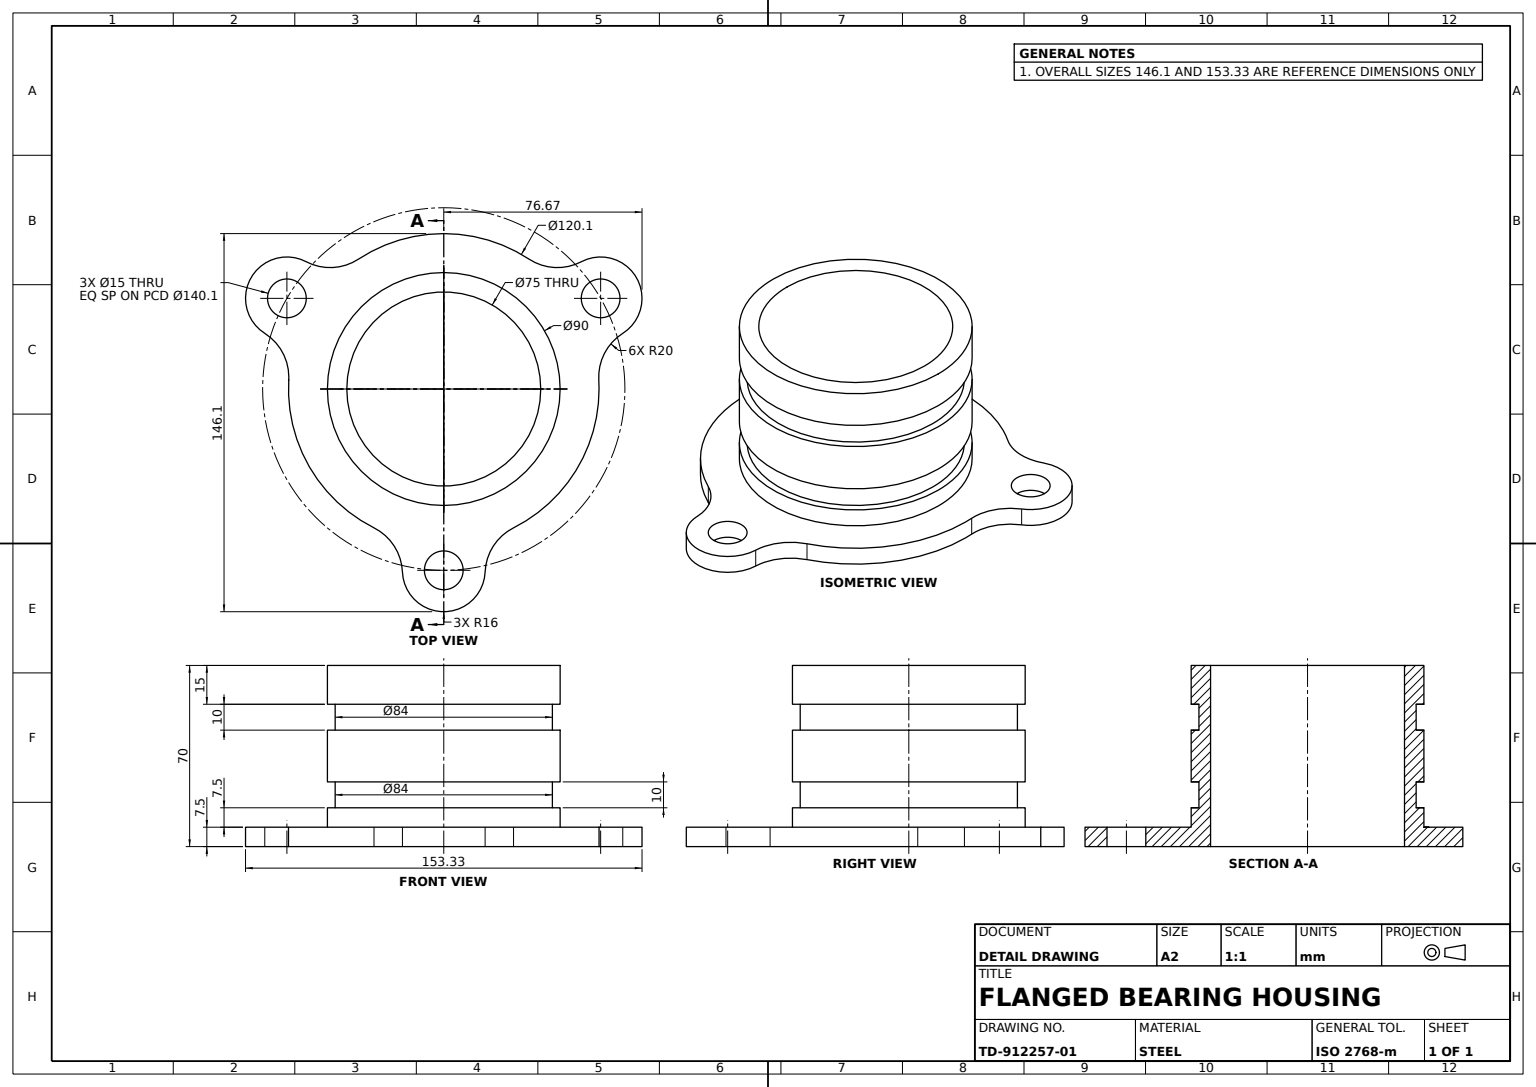
from build123d import *

# Parameters (mm, degrees)
MOUNTING_START               = -7.5
MOUNTING_FLANGE_SKETCH_R     = 37.5
MOUNTING_FLANGE_SKETCH_R_2   = 7.5
MOUNTING_FLANGE_3_LUGS_DEPTH = 7.5


with BuildPart() as part:
    # Housing Profile Sketch → Housing Sleeve Revolve (revolve)
    with BuildSketch(Plane.XY):
        Polygon((45, 0), (37.5, 0), (37.5, 70), (45, 70), (45, 55), (42, 55), (42, 45), (45, 45), (45, 25), (42, 25), (42, 15), (45, 15), align=None)
    revolve(axis=Axis((0, -100.894385012, 0), (0, 1, 0)))

    # Mounting Flange Sketch → Mounting Flange 3 Lugs (add)
    with BuildSketch(Plane.XZ.offset(MOUNTING_START)):
        with BuildLine():
            ThreePointArc((-26.98330478, 53.646097371), (-52.004825497, 30.025), (-59.950535527, -3.454821269))
            ThreePointArc((-59.950535527, -3.454821269), (-62.126875731, -13.743136068), (-69.221670101, -21.50520866))
            ThreePointArc((-69.221670101, -21.50520866), (-74.521485996, -43.025), (-53.234892064, -49.19512047))
            ThreePointArc((-53.234892064, -49.19512047), (-42.965342828, -46.931884607), (-32.967230748, -50.191276103))
            ThreePointArc((-32.967230748, -50.191276103), (0, -60.05), (32.967230748, -50.191276103))
            ThreePointArc((32.967230748, -50.191276103), (42.965342828, -46.931884607), (53.234892064, -49.19512047))
            ThreePointArc((53.234892064, -49.19512047), (74.521485996, -43.025), (69.221670101, -21.50520866))
            ThreePointArc((69.221670101, -21.50520866), (62.126875731, -13.743136068), (59.950535527, -3.454821269))
            ThreePointArc((59.950535527, -3.454821269), (52.004825497, 30.025), (26.98330478, 53.646097371))
            ThreePointArc((26.98330478, 53.646097371), (19.161532903, 60.675020674), (15.986778038, 70.70032913))
            ThreePointArc((15.986778038, 70.70032913), (0, 86.05), (-15.986778038, 70.70032913))
            ThreePointArc((-15.986778038, 70.70032913), (-19.161532903, 60.675020674), (-26.98330478, 53.646097371))
        make_face()
        Circle(MOUNTING_FLANGE_SKETCH_R, mode=Mode.SUBTRACT)
        with Locations((0, 70.05)):
            Circle(MOUNTING_FLANGE_SKETCH_R_2, mode=Mode.SUBTRACT)
        with Locations((60.665079535, -35.025)):
            Circle(MOUNTING_FLANGE_SKETCH_R_2, mode=Mode.SUBTRACT)
        with Locations((-60.665079535, -35.025)):
            Circle(MOUNTING_FLANGE_SKETCH_R_2, mode=Mode.SUBTRACT)
    extrude(amount=MOUNTING_FLANGE_3_LUGS_DEPTH)


solid = part.part
